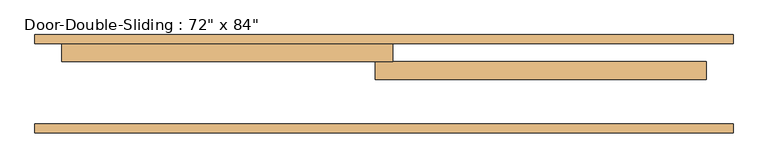
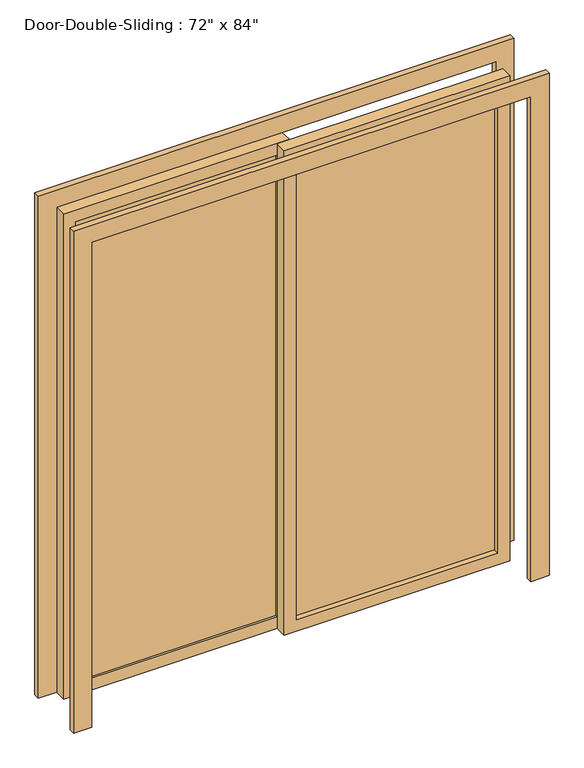
"""IFC4 building model written with IfcOpenShell, lengths in millimetres: door geometry."""

from ifc_helpers import new_model, si_unit, frame, origin, place, context, project, spatial, polyline, outline, extrude, source, transform, mapped, element, save


def door_d4d75d1e(model_context):
    return source(origin(), model_context, "Body", "SweptSolid", [
        extrude(outline(polyline([(0.0, 990.6), (2209.8, 990.6), (2209.8, -990.6), (0.0, -990.6), (0.0, -914.4), (2133.6, -914.4), (2133.6, 914.4), (0.0, 914.4), (0.0, 990.6)])), frame((0.0, 241.3, 0.0), z_axis=(0.0, 1.0, 0.0), x_axis=(0.0, 0.0, 1.0)), (0.0, 0.0, 1.0), 25.4),
        extrude(outline(polyline([(0.0, -990.6), (0.0, -914.4), (2133.6, -914.4), (2133.6, 914.4), (0.0, 914.4), (0.0, 990.6), (2209.8, 990.6), (2209.8, -990.6), (0.0, -990.6)])), frame((0.0, -12.7, 0.0), z_axis=(0.0, 1.0, 0.0), x_axis=(0.0, 0.0, 1.0)), (0.0, 0.0, 1.0), 25.4),
        extrude(outline(polyline([(2133.6, 25.4), (2133.6, -914.4), (0.0, -914.4), (0.0, 25.4), (2133.6, 25.4)]), holes=[polyline([(2082.8, -25.4), (50.8, -25.4), (50.8, -863.6), (2082.8, -863.6), (2082.8, -25.4)])]), frame((0.0, 190.5, 0.0), z_axis=(0.0, 1.0, 0.0), x_axis=(0.0, 0.0, 1.0)), (0.0, 0.0, 1.0), 50.8),
        extrude(outline(polyline([(2133.6, -25.4), (0.0, -25.4), (0.0, 914.4), (2133.6, 914.4), (2133.6, -25.4)]), holes=[polyline([(2082.8, 25.4), (2082.8, 863.6), (50.8, 863.6), (50.8, 25.4), (2082.8, 25.4)])]), frame((0.0, 139.7, 0.0), z_axis=(0.0, 1.0, 0.0), x_axis=(0.0, 0.0, 1.0)), (0.0, 0.0, 1.0), 50.8),
        extrude(outline(polyline([(-25.4, 200.025), (-863.6, 200.025), (-863.6, 206.375), (-25.4, 206.375), (-25.4, 200.025)])), frame((0.0, 0.0, 50.8), z_axis=(0.0, 0.0, 1.0), x_axis=(1.0, 0.0, 0.0)), (0.0, 0.0, 1.0), 2032.0),
        extrude(outline(polyline([(25.4, 168.275), (863.6, 168.275), (863.6, 161.925), (25.4, 161.925), (25.4, 168.275)])), frame((0.0, 0.0, 50.8), z_axis=(0.0, 0.0, 1.0), x_axis=(1.0, 0.0, 0.0)), (0.0, 0.0, 1.0), 2032.0),
    ])


if __name__ == "__main__":
    model = new_model("IFC4")
    model_context = context("Model", 3, world=origin())
    ifc_project = project(units=[si_unit("LENGTHUNIT", "METRE", prefix="MILLI")], contexts=[model_context])
    site = spatial("IfcSite", under=ifc_project)
    building = spatial("IfcBuilding", under=site)
    placement = place(None, origin())
    door_shape = door_d4d75d1e(model_context)
    element("IfcDoor", 1, ObjectType="Door-Double-Sliding : 72\" x 84\"", at=placement, inside=building, context=model_context, shape_type="MappedRepresentation", body=[
        mapped(door_shape, transform((0.0, 0.0, 0.0), x_axis=(1.0, 0.0, 0.0), y_axis=(0.0, 1.0, 0.0), z_axis=(0.0, 0.0, 1.0))),
    ])
    save(model, "model.ifc")

# Revit data of these elements
# Type "Door-Double-Sliding : 72\" x 84\""
#   Type Mark = "13"
#   Construction Type Id = "opn-d45"
#   Assembly Code = "C1020"
#   Analytic Construction = "Wood frame, double glass door "
#   Thickness = 0' - 2"
#   Thermal Resistance (R) = 1.8150 (h·ft²·°F)/BTU
#   Heat Transfer Coefficient (U) = 0.5510 BTU/(h·ft²·°F)
#   Height = 7' - 0"
#   Rail Width = 0' - 2"
#   Stiles = 0' - 2"
#   Trim Projection Ext = 0' - 1"
#   Trim Projection Int = 0' - 1"
#   Trim Width = 0' - 3"
#   Width = 6' - 0"
#   Define Thermal Properties by = 1
#   Glazing = Glass
#   Panel Material = Wood - Birch - Solid Stained Light Low Gloss
#   Trim Material = Paint - Sienna
#   Visual Light Transmittance = 0
#   Solar Heat Gain Coefficient = 0
#   Function = (empty or 0)
#   Wall Closure = (empty or 0)
# Element 1 (IfcDoor, "Door-Double-Sliding : 72\" x 84\"")
#   Materials on its faces: "Paint - Sienna", "Wood - Birch - Solid Stained Light Low Gloss", "Glass"
# Materials
#   "Glass": class "Glass", colour RGB 0 128 192, transparency 0.75, Description = "Soda Lime Glass", Cost = 0
#   "Wood - Birch - Solid Stained Light Low Gloss": class "Wood", colour RGB 210 159 95, transparency 0, Cost = 0
#   "Paint - Sienna": colour RGB 118 70 51, transparency 0, Cost = 0
